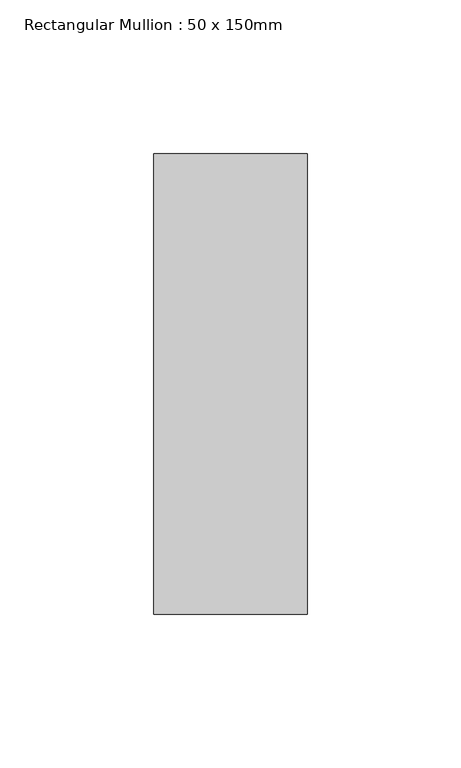
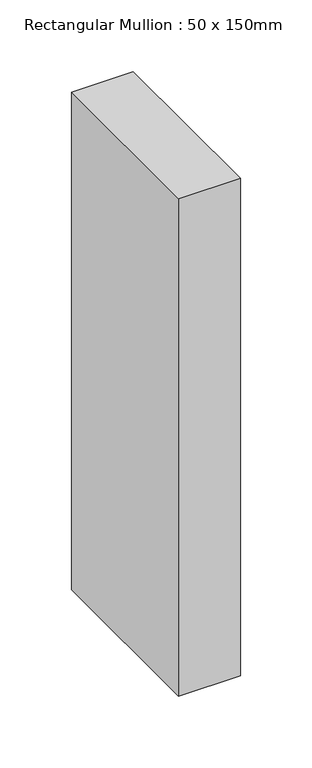
"""IFC4 building model written with IfcOpenShell, lengths in millimetres: member geometry, Rectangular Mullion : 50 x 150mm."""

from ifc_helpers import new_model, si_unit, frame, origin, place, context, project, spatial, polyline, outline, extrude, source, transform, mapped, element, save


def rectangular_mullion_50_x_150mm_89c22e8d(model_context):
    return source(origin(), model_context, "Body", "SweptSolid", [
        extrude(outline(polyline([(0.0, 75.0), (0.0, -75.0), (-50.0, -75.0), (-50.0, 75.0), (0.0, 75.0)])), frame((0.0, 0.0, -425.0), z_axis=(0.0, 0.0, 1.0), x_axis=(1.0, 0.0, 0.0)), (0.0, 0.0, 1.0), 425.0),
    ])


if __name__ == "__main__":
    model = new_model("IFC4")
    model_context = context("Model", 3, world=origin())
    ifc_project = project(units=[si_unit("LENGTHUNIT", "METRE", prefix="MILLI")], contexts=[model_context])
    site = spatial("IfcSite", under=ifc_project)
    building = spatial("IfcBuilding", under=site)
    placement = place(None, origin())
    rectangular_mullion_50_x_150mm_shape = rectangular_mullion_50_x_150mm_89c22e8d(model_context)
    element("IfcMember", 1, ObjectType="Rectangular Mullion : 50 x 150mm", at=placement, inside=building, context=model_context, shape_type="MappedRepresentation", body=[
        mapped(rectangular_mullion_50_x_150mm_shape, transform((0.0, 0.0, 0.0), x_axis=(1.0, 0.0, 0.0), y_axis=(0.0, 1.0, 0.0), z_axis=(0.0, 0.0, 1.0))),
    ])
    save(model, "model.ifc")

# Revit data of these elements
# Type "Rectangular Mullion : 50 x 150mm"
#   built-in parameter 1007304 = 0.492126 (stored number, unit not read)
#   built-in parameter 1007301 = 0.082021 (stored number, unit not read)
#   built-in parameter 1007300 = 0.082021 (stored number, unit not read)
# Element 1 (IfcMember, "Rectangular Mullion : 50 x 150mm")
#   Materials on its faces: "Aluminium"
# Materials
#   "Aluminium": class "Metal", colour RGB 247 247 247, transparency 0, Description = "Aluminium 6061", Cost = 0
